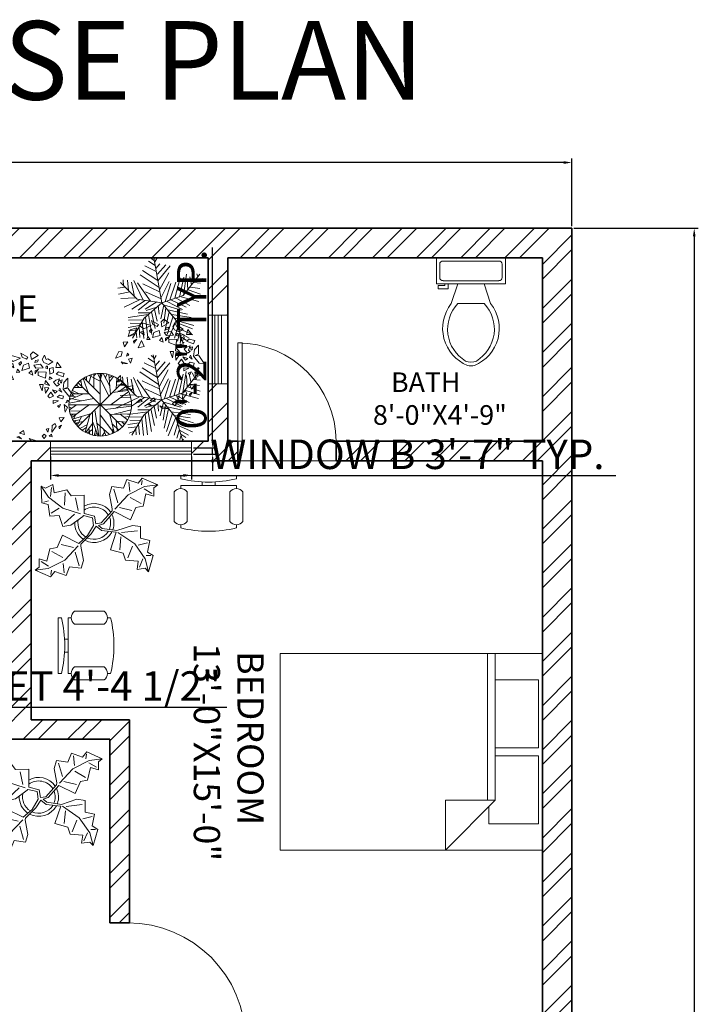
# Model space of a CAD drawing. Units: inches. Extents: x 744 to 1448, y 5126 to 6077.
# Tile 10 of 10: x 1152 to 1359, y 5585 to 5885. Entities that reach past the tile are written whole.
import ezdxf

# ---------------------------------------------------------------- set-up
doc = ezdxf.new("R2010")
doc.units = ezdxf.units.IN
for name, color, linetype, lineweight in [('A-ANNO-DIMS', 2, 'Continuous', 18), ('A-ANNO-TEXT', 7, 'Continuous', 18), ('A-AREA-IDEN', 7, 'Continuous', 18), ('A-DOOR', 4, 'Continuous', 18), ('A-FLOR-FIXT', 9, 'Continuous', 18), ('A-FURN', 8, 'Continuous', 18), ('A-WALL', 7, 'Continuous', 35), ('A-WALL-PATT', 252, 'Continuous', 13), ('L-PLNT', 3, 'Continuous', 13)]:
    doc.layers.add(name, color=color, linetype=linetype, lineweight=lineweight)
doc.layers.add('A-GLAZ', color=244, linetype='Continuous', lineweight=18, true_color=0x991b1e)
doc.styles.get("Standard").update_dxf_attribs({"font": 'arial.ttf'})
doc.dimstyles.new('ISO-25', dxfattribs={"dimtxt": 9, "dimasz": 2.5, "dimexe": 1.25, "dimexo": 0.625, "dimtad": 1, "dimlunit": 3, "dimtxsty": 'Standard', "dimcen": 2.5, "dimadec": 0, "dimazin": 0, "dimtfac": 1, "dimtmove": 0, "dimatfit": 3, "dimfxl": 1, "dimarcsym": 0})

# ---------------------------------------------------------------- blocks, each defined once
blk = doc.blocks.new('*U5')
for p, q in [((0, 0), (0, 6)), ((40, 0), (40, 6))]:
    blk.add_line(p, q)
blk.add_lwpolyline([(0, 0), (0, -40), (1.75, -40), (1.75, 0)], close=True)
blk.add_arc((0, 0), 40, 270, 0)
blk = doc.blocks.new('*U3')
for p, q in [((-40, 0), (-40, 6)), ((0, 0), (0, 6))]:
    blk.add_line(p, q)
blk.add_lwpolyline([(0, 0), (0, -40), (-1.75, -40), (-1.75, 0)], close=True)
blk.add_arc((0, 0), 40, 180, 270)
blk = doc.blocks.new('*U8')
for p, q in [((9.5, -6), (9.5, -2)), ((-10, -8.5), (-8, -8.5)), ((-10, -9.5), (-10, -8.5)), ((-8, -8.5), (-8, -8)), ((-7, -8), (-7, -9.5)), ((-4, -8), (-6, -14)), ((4, -8), (6, -14)), ((-7, -9.5), (-10, -9.5)), ((4, -14), (-4, -14))]:
    blk.add_line(p, q)
blk.add_lwpolyline([(10.5, -8), (10.5, 0), (-10.5, 0), (-10.5, -8)], close=True)
for points in [[(-9.5, -2), (-9.5, -6)], [(8.5, -1), (-8.5, -1)], [(-8.5, -7), (8.5, -7)]]:
    blk.add_lwpolyline(points)
for centre, radius, start, end in [((-8.62, -1.88), 0.884, 81.8699, 188.1301), ((8.62, -1.88), 0.884, 351.8699, 98.1301), ((-8.62, -6.12), 0.884, 171.8699, 278.1301), ((8.62, -6.12), 0.884, 261.8699, 8.1301), ((3.52, -21.58), 12.17, 141.4691, 247.9714), ((4.2, -21.82), 11.33, 136.3677, 238.9468), ((-3.52, -21.58), 12.17, 292.0284, 38.5307), ((-4.2, -21.82), 11.33, 301.053, 43.6321), ((0, -27.88), 4, 245.7318, 294.2682), ((0, -29), 4, 254.8605, 285.1395)]:
    blk.add_arc(centre, radius, start, end)
blk = doc.blocks.new('Bed - Queen')
for p, q in [((0, -80.00003), (0, 0)), ((0, 0), (59.99999, 0)), ((59.99999, 0), (59.99999, -80.00003)), ((7.99999, -1.2), (28.79998, -1.2)), ((7.99999, -14.4), (7.99999, -1.2)), ((28.79998, -1.2), (28.79998, -14.4)), ((31.19999, -1.2), (51.99999, -1.2)), ((31.19999, -14.4), (31.19999, -1.2)), ((51.99999, -1.2), (51.99999, -16.4)), ((0, -14.4), (44.8, -14.4)), ((59.99999, -29.6), (44.8, -14.4)), ((44.8, -14.4), (44.8, -29.6)), ((44.8, -16.8), (0, -16.8)), ((51.99999, -16.4), (46.79936, -16.4)), ((44.8, -29.6), (59.99999, -29.6)), ((59.99999, -80.00003), (0, -80.00003))]:
    blk.add_line(p, q)
blk = doc.blocks.new('Plant - Rubber or Philodendron')
for p, q in [((8.8871, 10.7908), (9.9809, 13.4933)), ((9.9809, 13.4933), (13.3837, 12.301)), ((10.5828, 12.6946), (10.8893, 9.7953)), ((13.3837, 12.301), (14.68, 13.9039)), ((14.5816, 13.2037), (14.3848, 11.8033)), ((14.68, 13.9039), (19.3848, 11.8146)), ((-16.2005, 11.4774), (-13.9899, 8.1064)), ((-16.2005, 11.4774), (-14.8639, 10.7964)), ((-16.0159, 6.3329), (-16.2005, 11.4774)), ((-14.8639, 10.7964), (-12.6195, 11.8975)), ((-13.3174, 8.325), (-13.0735, 11.0065)), ((-12.6195, 11.8975), (-12.1909, 9.4345)), ((-12.1909, 9.4345), (-8.3829, 10.3)), ((-8.8369, 9.409), (-9.0894, 5.6095)), ((-8.3829, 10.3), (-7.0549, 8.501)), ((4.6914, 8.8812), (5.3859, 11.2828)), ((5.3859, 11.2828), (8.8871, 10.7908)), ((5.9878, 10.4842), (7.1971, 6.3869)), ((15.3859, 11.3055), (10.3916, 8.7942)), ((15.7909, 9.1065), (14.8995, 5.3044)), ((15.2875, 10.6053), (17.5907, 9.2105)), ((19.3848, 11.8146), (15.3859, 11.3055)), ((18.1925, 8.4119), (15.7909, 9.1065)), ((19.3848, 11.8146), (18.1868, 10.9119)), ((18.1868, 10.9119), (18.1925, 8.4119)), ((-14.0069, 5.8704), (-16.0159, 6.3329)), ((-15.3434, 6.5514), (-13.9984, 6.9884)), ((-13.9899, 8.1064), (-9.5434, 4.7185)), ((-7.0549, 8.501), (-3.0284, 8.6941)), ((-4.8529, 4.012), (-5.7184, 7.82)), ((-3.0284, 8.6941), (-3.0709, 3.1041)), ((4.6914, 8.8812), (5.5014, 4.4831)), ((10.3916, 8.7942), (6.2847, 4.4028)), ((14.2977, 6.1031), (10.9934, 7.9956)), ((-13.5868, 2.2894), (-14.0069, 5.8704)), ((-13.1329, 3.1804), (-10.6614, 4.727)), ((-9.5434, 4.7185), (-4.1917, 2.9888)), ((-3.0709, 3.1041), (0.0797, 2.3163)), ((2.1141, 0.2298), (5.4346, 3.9146)), ((6.1032, 3.6844), (2.8262, -0.031)), ((5.4346, 3.9146), (5.5014, 4.4831)), ((11.1089, 1.1958), (6.1032, 3.6844)), ((7.7005, 4.8881), (11.5025, 3.9967)), ((12.7005, 4.8994), (11.1089, 1.1958)), ((14.8995, 5.3044), (12.7005, 4.8994)), ((-10.6784, 2.491), (-13.5868, 2.2894)), ((-9.5858, -0.8715), (-10.6784, 2.491)), ((-9.1318, 0.0195), (-5.9793, 2.9025)), ((-7.1228, -0.443), (-3.5248, 2.2131)), ((-3.5248, 2.2131), (-3.3011, 2.4355)), ((-3.3011, 2.4355), (-0.5306, 1.7947)), ((-0.5306, 1.7947), (-0.2255, -0.5527)), ((-0.5306, 1.7947), (-0.5306, 1.7947)), ((0.0797, 2.3163), (0.4866, -0.031)), ((0.4866, -0.031), (2.1141, 0.2298)), ((-7.1228, -0.443), (-9.5858, -0.8715)), ((-2.019, -3.6148), (-0.2255, -0.5527)), ((-0.9375, -3.1608), (0.5883, -0.8135)), ((0.5883, -0.8135), (2.2447, -2.0916)), ((2.8262, -0.031), (1.3003, -0.5527)), ((1.3003, -0.5527), (2.4193, -1.4655)), ((2.2447, -2.0916), (6.7108, -2.6626)), ((2.4193, -1.4655), (6.895, -2.1175)), ((4.943, -7.9659), (6.7108, -2.6626)), ((11.6605, -0.5413), (6.895, -2.1175)), ((12.3677, -6.1981), (7.219, -2.6772)), ((8.3544, -2.7453), (13.1973, -2.1704)), ((11.6605, -0.5413), (14.1354, -0.8948)), ((14.1354, -0.8948), (14.1354, -4.4304)), ((-11.3237, -7.2629), (-9.7321, -3.5593)), ((-9.7321, -3.5593), (-4.7264, -6.0479)), ((-2.019, -3.6148), (-4.7264, -6.0479)), ((-4.0579, -6.2781), (-0.9375, -3.1608)), ((8.125, -4.0768), (7.7715, -7.9659)), ((16.2567, -5.8446), (13.4283, -6.5517)), ((14.1354, -4.4304), (16.9638, -5.1375)), ((16.9638, -5.1375), (16.2567, -8.673)), ((-14.4141, -11.4699), (-13.5228, -7.6679)), ((-13.5228, -7.6679), (-11.3237, -7.2629)), ((-12.921, -8.4665), (-9.6166, -10.359)), ((-6.3237, -7.2516), (-10.1257, -6.3602)), ((-9.0148, -11.1577), (-4.9047, -6.8122)), ((-4.611, -12.8477), (-5.8203, -8.7504)), ((-4.1246, -6.8466), (-4.0579, -6.2781)), ((-3.3146, -11.2447), (-4.1246, -6.8466)), ((8.8321, -9.0266), (4.943, -7.9659)), ((10.2463, -10.4408), (11.6605, -6.9053)), ((15.5496, -10.7943), (12.3677, -6.1981)), ((16.2567, -8.673), (18.0245, -9.7337)), ((-16.8157, -10.7754), (-14.4141, -11.4699)), ((-16.8101, -13.2754), (-16.8157, -10.7754)), ((-13.9107, -12.9688), (-16.2139, -11.574)), ((-14.0091, -13.669), (-9.0148, -11.1577)), ((-3.3146, -11.2447), (-4.0092, -13.6463)), ((9.5392, -11.1479), (8.8321, -9.0266)), ((13.4283, -11.5015), (9.5392, -11.1479)), ((13.0748, -13.9763), (13.4283, -11.5015)), ((14.8425, -10.7943), (13.7819, -13.2692)), ((16.6103, -14.6834), (15.5496, -10.7943)), ((17.3174, -9.7337), (15.9032, -9.7337)), ((18.0245, -9.7337), (16.6103, -14.6834)), ((-18.008, -14.1781), (-16.8101, -13.2754)), ((-18.008, -14.1781), (-14.0091, -13.669)), ((-13.3032, -16.2674), (-18.008, -14.1781)), ((-12.0069, -14.6645), (-13.3032, -16.2674)), ((-13.2048, -15.5672), (-13.008, -14.1668)), ((-8.6042, -15.8568), (-12.0069, -14.6645)), ((-9.206, -15.0581), (-9.5126, -12.1588)), ((-7.5103, -13.1543), (-8.6042, -15.8568)), ((-4.0092, -13.6463), (-7.5103, -13.1543)), ((15.5496, -13.6228), (13.0748, -13.9763)), ((16.6103, -14.6834), (15.5496, -13.6228))]:
    blk.add_line(p, q)
for centre, radius, start, end in [((0, 0), 6.1275, 34.37569, 120.1028), ((-0.0601, -0.2075), 5.2461, 33.82192, 124.9414), ((0.0308, 0.1664), 6, 178.6147, 235.1169), ((0.0308, 0.1664), 5, 168.1647, 238.6725), ((-0.2664, 0.1682), 5.2775, 338.4094, 20.03007), ((-0.098, 0.1364), 6.1288, 341.2017, 26.09184), ((-0.0234, 0.3825), 6.1492, 242.5812, 331.2714), ((-0.1102, 0.4886), 5.2883, 247.3711, 327.472)]:
    blk.add_arc(centre, radius, start, end)
blk = doc.blocks.new('*U11')
for points in [[(-4.43, 11.05), (-5.18, 10.36), (-3.96, 9.49), (-2.07, 10.36)], [(-2, 11.66), (-1.6, 10.62), (-0.52, 10.1), (-0.18, 10.62), (-0.79, 10.96)], [(1.24, 12), (0.56, 11.31), (0.76, 10.01), (2.52, 11.05)], [(4.14, 11.14), (3.6, 10.01), (4, 9.23), (5.22, 8.71), (6.3, 9.41), (5.08, 10.19), (4.61, 10.01)], [(-5.78, 9.75), (-7.54, 9.23), (-8.01, 7.5), (-6.26, 8.45)], [(-4.84, 8.63), (-3.83, 7.85), (-4.03, 8.97)], [(-1.94, 9.49), (-2.48, 8.97), (-2.27, 8.54), (-1.8, 9.06)], [(0.02, 9.06), (-1.33, 8.54), (-1.73, 7.16), (0.29, 7.76)], [(1.37, 8.54), (3.13, 8.8), (3.8, 7.85), (1.91, 7.76)], [(2.59, 9.93), (1.84, 9.75), (1.64, 9.23), (2.32, 9.41)], [(4.61, 8.28), (4.54, 7.76), (4.95, 7.59), (4.95, 8.28)], [(6.43, 7.94), (5.49, 7.68), (5.56, 6.21), (6.5, 6.64)], [(7.45, 9.32), (7.11, 7.94), (8.52, 7.94)], [(-8.14, 6.03), (-9.36, 5.95), (-9.02, 4.73)], [(-5.78, 6.81), (-6.66, 6.21), (-6.52, 5.69)], [(-4.57, 6.38), (-5.45, 4.47), (-3.89, 4.82)], [(-2.88, 7.5), (-3.15, 6.64), (-2.27, 6.72)], [(0.76, 7.16), (0.09, 6.46), (1.1, 5.95)], [(1.71, 6.29), (1.71, 7.07), (2.65, 7.5), (2.11, 6.9)], [(2.52, 6.81), (2.52, 5.86), (4.41, 5.17), (4.61, 6.72)], [(5.49, 5.51), (5.42, 4.82), (6.16, 5.08)], [(7.85, 6.81), (7.18, 6.21), (9, 5.51), (9.33, 6.38)], [(10.28, 5.17), (9.2, 4.04), (9, 2.31), (10.48, 0.49), (11.76, 0.41), (10.35, 2.48), (9.33, 2.4), (10.28, 2.83)], [(-11.32, 1.79), (-9.83, 2.31), (-9.63, 3.44), (-10.44, 3.52)], [(-8.21, 3.09), (-8.48, 2.31), (-7.87, 2.57)], [(3.53, 1.88), (2.86, 3.52), (3.8, 3.52)], [(4.41, 4.56), (4.27, 3.7), (5.49, 3.26)], [(4.27, 2.74), (5.29, 2.66), (4.41, 1.27)], [(8.12, 4.99), (7.11, 4.65), (6.5, 4.13), (7.38, 3.09), (8.12, 3.52), (7.65, 3.87)], [(8.19, 2.57), (7.92, 2.05), (8.66, 1.53)], [(8.73, 4.73), (8.19, 4.56), (8.39, 3.87), (8.59, 4.04)], [(-8.21, 0.41), (-9.43, 0.32), (-9.83, 0.84)], [(-7, 1.79), (-7.94, 1.53), (-7.47, 0.49)], [(5.83, 1.53), (5.02, 0.41), (5.49, -0.02), (6.5, 0.41)], [(7.51, 1.71), (6.91, 1.27), (6.23, 2.14)], [(8.12, 0.75), (7.51, 0.15), (8.93, -0.28), (9.13, 0.49)], [(7.78, -0.8), (6.43, -1.5), (6.43, -0.72)], [(8.32, -1.75), (7.98, -2.53), (7.58, -2.1)], [(9.33, -1.75), (9.54, -3.74), (10.14, -2.53)], [(10.08, -0.63), (9.74, -1.32), (10.48, -0.89)], [(-10.03, -2.71), (-10.64, -3.31), (-10.44, -4.44), (-9.9, -3.49)], [(-8.28, -5.73), (-6.79, -5.3), (-7, -6.51)], [(6.1, -8.94), (6.16, -7.21), (6.91, -6.69), (7.24, -7.38)], [(8.05, -8.07), (8.59, -7.12), (7.92, -7.55)], [(9.33, -5.13), (8.46, -6.25), (7.98, -5.22)], [(-4.84, -8.85), (-4.43, -9.45), (-5.99, -9.8)], [(-2.54, -10.06), (-3.02, -10.23), (-1.8, -10.67)], [(-2.34, -9.2), (-1.26, -8.5), (-0.99, -9.54)], [(4.07, -9.45), (3.53, -9.97), (4.07, -10.58), (4.61, -9.89)], [(5.29, -7.98), (4.61, -8.16), (5.02, -8.94)], [(6.03, -9.45), (5.42, -9.97), (6.16, -10.15)], [(0.22, -10.58), (0.83, -11.27), (2.59, -11.36)]]:
    blk.add_lwpolyline(points, close=True)
blk = doc.blocks.new('*U10')
for p, q in [((-8.737, 47.138), (-17.069, 52.711)), ((-10.186, 53.64), (-13.084, 55.962)), ((0, 0), (-10.5, 57)), ((-9.099, 51.782), (-6.563, 55.962)), ((-5.114, 28.097), (-24.676, 40.636)), ((-7.288, 39.707), (-21.778, 46.673)), ((-7.65, 43.423), (-2.578, 49.46)), ((-5.839, 35.992), (4.667, 48.067)), ((-5.114, 27.632), (10.463, 46.673)), ((-2.941, 16.486), (8.652, 37.85)), ((-31.5, 4.5), (-52.5, 25.5)), ((-48.585, 21.131), (-49.309, 29.026)), ((-43.513, 28.561), (-42.427, 15.558)), ((-38.442, 26.239), (-34.819, 7.663)), ((-35.544, 28.097), (-24.314, 3.947)), ((-14.533, 2.09), (-30.834, 25.31)), ((-3.665, 19.273), (-27.574, 35.527)), ((-1.129, 6.734), (9.014, 26.704)), ((10.101, 3.483), (17.708, 26.239)), ((16.259, 5.805), (23.142, 31.348)), ((22.055, 7.198), (27.489, 32.277)), ((27, 9), (48, 36)), ((27.127, 9.056), (31.112, 35.992)), ((31.836, 30.883), (32.561, 16.486)), ((35.096, 32.741), (37.27, 22.524)), ((38.719, 34.134), (41.979, 28.561)), ((40.53, 25.775), (48.862, 24.846)), ((43.791, 29.954), (51.036, 30.883)), ((44.153, 36.456), (45.239, 32.741)), ((-47.498, 19.737), (-55.83, 18.344)), ((-40.615, 13.7), (-55.105, 10.913)), ((-24.314, 23.917), (-2.941, 13.7)), ((-20.691, 13.7), (-1.129, 4.876)), ((3.942, 1.625), (11.187, 24.381)), ((33.285, 16.486), (48.862, 10.913)), ((36.183, 19.737), (48.137, 17.88)), ((-33.37, 6.269), (-52.207, 5.34)), ((-28.299, 3.483), (-47.86, -5.805)), ((-21.416, 3.018), (-38.079, -8.128)), ((0, 0), (-31.5, 4.5)), ((-15.982, 2.09), (-30.11, -9.521)), ((0, 0), (-22.5, -19.5)), ((-6.563, 1.161), (-21.416, -8.128)), ((0, 0), (27, 9)), ((0, 0), (18, -22.5)), ((6.478, 1.625), (26.04, -8.592)), ((11.187, 3.483), (30.749, -5.805)), ((18.07, 5.805), (35.096, -3.483)), ((24.229, 7.663), (46.688, 1.625)), ((29.662, 12.307), (48.137, 6.269)), ((-6.563, -5.805), (-19.967, -9.985)), ((-13.446, -11.378), (-8.737, -32.741)), ((-9.461, -8.592), (-6.201, -23.453)), ((-4.752, -3.483), (-3.665, -14.629)), ((2.493, -3.019), (-1.491, -20.202)), ((1.769, -2.555), (24.229, -9.521)), ((5.029, -6.27), (2.131, -25.775)), ((9.014, -11.378), (3.58, -35.992)), ((7.565, -9.056), (32.198, -14.629)), ((-17.431, -15.094), (-42.789, -18.809)), ((-24.314, -21.596), (-42.427, -22.06)), ((-22.5, -19.5), (-37.5, -45)), ((-15.257, -12.772), (-30.11, -12.772)), ((-25.038, -23.918), (-22.865, -45.281)), ((-20.691, -18.345), (-17.793, -44.352)), ((-17.069, -15.094), (-12.721, -40.172)), ((14.085, -16.951), (6.478, -40.172)), ((18.07, -22.524), (8.289, -45.745)), ((12.274, -15.094), (36.907, -18.809)), ((16.259, -19.738), (36.183, -22.989)), ((18, -22.5), (27, -52.5)), ((18.433, -22.524), (40.53, -29.026)), ((-28.299, -29.026), (-42.789, -31.348)), ((-30.834, -34.135), (-42.427, -35.528)), ((-26.849, -26.24), (-40.253, -25.775)), ((-32.646, -36.921), (-31.921, -44.352)), ((-29.023, -30.884), (-27.936, -43.887)), ((20.244, -30.419), (15.897, -44.816)), ((19.157, -25.311), (38.719, -33.206)), ((21.331, -32.741), (39.081, -40.636)), ((-34.457, -39.708), (-40.978, -42.494)), ((22.78, -37.85), (19.519, -48.532)), ((22.78, -38.314), (34.372, -44.816)), ((24.591, -45.745), (23.142, -50.854)), ((24.591, -43.423), (30.749, -47.603)), ((26.764, -49.925), (28.213, -50.854))]:
    blk.add_line(p, q)
blk = doc.blocks.new('*U13')
for p, q in [((-22.0458, 42.0753), (-16.5881, 57.6486)), ((-12.5388, 54.9406), (-7.9613, 59.4546)), ((-12.3627, 32.1443), (-12.5388, 58.7776)), ((-5.3205, 59.6806), (16.5105, 16.7963)), ((2.426, 54.9406), (-1.4472, 59.9056)), ((0, 59.9996), (0, -60)), ((0.4894, 48.6208), (3.6584, 59.6806)), ((18.2711, 35.5298), (5.419, 59.6806)), ((9.8203, 51.5549), (12.8133, 58.5516)), ((19.6795, 19.5047), (16.3344, 57.6486)), ((-45.8134, 38.2383), (-40.5318, 33.0471)), ((-43.8768, 36.4326), (-44.405, 40.2696)), ((42, 42), (-42, -42)), ((42, -42), (-42, 42)), ((-40.1797, 44.558), (-36.4825, 43.2038)), ((-37.0107, 47.0408), (-35.25, 35.5298)), ((-32.6092, 50.4264), (-23.2782, 23.5674)), ((-31.2008, 51.1035), (-0.2149, 20.1818)), ((-26.4472, 46.5894), (-26.2712, 53.8116)), ((-21.1656, 55.8436), (-0.0388, 45.0094)), ((17.0387, 51.1035), (23.2006, 55.1666)), ((17.7429, 43.6552), (25.4894, 54.2636)), ((31.6513, 50.8778), (30.2429, 30.5643)), ((31.1232, 42.5267), (35.8767, 48.1693)), ((-32.2571, 20.6333), (-59.1937, 9.348)), ((-56.0247, 20.859), (-20.8134, 20.859)), ((-54.7923, 24.4702), (-47.75, 21.0847)), ((-53.2078, 27.4044), (-40.1797, 20.859)), ((-49.8627, 32.8214), (-32.7853, 32.8214)), ((54.3626, 25.3731), (20.9119, 0.3198)), ((23.3767, 23.3417), (53.3063, 27.4044)), ((36.2288, 25.1474), (48.9049, 35.0784)), ((37.1091, 37.1098), (46.6161, 37.5612)), ((-59.7219, 2.8025), (-12.0106, 12.0565)), ((-58.6656, 12.7336), (-35.9543, 7.5424)), ((-57.081, 17.9248), (-47.0458, 14.7649)), ((-54.6162, -24.7335), (-20.2853, 0.0941)), ((29.3626, -6.6771), (59.4682, 7.091)), ((38.5175, 13.4107), (58.2359, 13.6364)), ((-60, 0), (60, 0)), ((-59.7219, -4.8714), (-54.2641, -6.6771)), ((-45.2853, -0.1316), (-59.0177, -10.0627)), ((-58.4895, -12.3197), (-36.4825, -11.6426)), ((-57.081, -18.4138), (-45.2853, -17.9624)), ((-52.6797, -18.188), (-55.4966, -22.0251)), ((-53.2078, -27.442), (-16.7641, -16.6081)), ((-14.8275, -15.0282), (-14.6515, -57.6865)), ((-10.074, -10.0627), (-2.5036, -59.7178)), ((9.2922, -9.1598), (59.6443, -2.8401)), ((18.6232, -18.6394), (26.7218, -53.3981)), ((18.7992, -18.6394), (57.3556, -17.2853)), ((26.3697, -18.4138), (58.9401, -9.8369)), ((38.1654, -18.188), (52.426, -29.0219)), ((-38.9472, -29.0219), (-51.4472, -30.6018)), ((-47.2219, -19.3166), (-50.2148, -26.3135)), ((-46.5177, -30.1504), (-49.5106, -33.536)), ((-32.4331, -32.4075), (-48.1021, -35.5674)), ((-43.7008, -34.6645), (-46.6937, -37.373)), ((-35.9543, -22.4765), (-44.0529, -40.5329)), ((-19.9331, -20.2194), (-28.5599, -52.721)), ((-14.6515, -36.2445), (-27.6797, -52.9467)), ((-14.6515, -32.1818), (-3.912, -59.4922)), ((-6.2008, -36.2445), (17.919, -57.0094)), ((-0.0388, -19.0909), (25.8415, -53.8495)), ((22.8485, -36.4702), (35.3485, -48.4326)), ((30.419, -30.1504), (32.3556, -50.0125)), ((31.4753, -31.279), (49.6091, -33.3103)), ((41.5105, -32.6332), (46.088, -38.0501)), ((45.9119, -24.0564), (55.595, -22.2508)), ((-24.6867, -37.8244), (-38.7712, -45.7241)), ((-26.2712, -43.9185), (-34.7219, -48.6583)), ((-14.6515, -47.3041), (-25.0388, -54.3009)), ((-21.5177, -45.4984), (-19.9331, -56.1065)), ((-8.4895, -47.5298), (-11.4825, -58.5893)), ((-6.3768, -52.721), (-9.3698, -58.815)), ((8.4119, -53.1724), (3.8344, -59.4922)), ((5.9471, -46.6269), (10.5246, -58.5893)), ((24.7852, -44.8213), (23.0246, -54.978))]:
    blk.add_line(p, q)
blk.add_circle((0, 0), 60)
blk = doc.blocks.new('Chair - Desk')
for p, q in [((-8.5, 0), (-8.5, -1)), ((-8.5, 0), (8.5, 0)), ((8.5, 0), (8.5, -1)), ((-8.5, -3), (-8.5, -4)), ((-8.5, -3), (8.5, -3)), ((-2, -3), (-2, -1.9355)), ((2, -1.9576), (2, -3)), ((8.5, -3), (8.5, -4)), ((-10.5, -5), (-10.5, -14)), ((-6.5, -14), (-6.5, -5)), ((6.5, -5), (6.5, -14)), ((10.5, -14), (10.5, -5)), ((-8.5, -15), (-8.5, -16)), ((8.5, -15), (8.5, -16))]:
    blk.add_line(p, q)
for centre, radius, start, end in [((0, 34.625), 36.625, 256.5803, 283.4197), ((-8.5, -6.5), 2.5, 36.8699, 143.1301), ((8.5, -6.5), 2.5, 36.8699, 143.1301), ((-8.5, -12.5), 2.5, 216.8699, 323.1301), ((8.5, -12.5), 2.5, 216.8699, 323.1301), ((0, 19.625), 36.625, 256.5803, 283.4197)]:
    blk.add_arc(centre, radius, start, end)
blk = doc.blocks.new('*D23')
at = {"layer": 'A-ANNO-DIMS', "color": 0, "lineweight": -2, "transparency": 16777216}
for p, q in [((1321.31, 5821.82), (1359.26, 5821.82)), ((1358.01, 5819.32), (1358.01, 5252.82)), ((1321.31, 5250.32), (1359.26, 5250.32))]:
    blk.add_line(p, q, dxfattribs=at)
at = {"layer": 'A-ANNO-DIMS', "color": 0, "transparency": 16777216}
for points in [[(1357.59, 5819.32), (1358.42, 5819.32), (1358.01, 5821.82)], [(1357.59, 5252.82), (1358.42, 5252.82), (1358.01, 5250.32)]]:
    blk.add_solid(points, dxfattribs=at)
at = {"layer": 'Defpoints', "color": 0, "transparency": 16777216}
for p in [(1320.68, 5821.82), (1320.68, 5250.32), (1358.01, 5250.32)]:
    blk.add_point(p, dxfattribs=at)
at = {"layer": 'A-ANNO-DIMS', "color": 0, "transparency": 16777216, "insert": (1352.81, 5536.07), "char_height": 9, "attachment_point": 5, "rotation": 90}
blk.add_mtext('47\'-7.5"', dxfattribs=at)
blk = doc.blocks.new('*D24')
at = {"layer": 'A-ANNO-DIMS', "color": 0, "lineweight": -2, "transparency": 16777216}
for p, q in [((804.68, 5822.44), (804.68, 5843.13)), ((1320.68, 5822.44), (1320.68, 5843.13)), ((1318.18, 5841.88), (807.18, 5841.88))]:
    blk.add_line(p, q, dxfattribs=at)
at = {"layer": 'A-ANNO-DIMS', "color": 0, "transparency": 16777216}
for points in [[(807.18, 5842.3), (807.18, 5841.46), (804.68, 5841.88)], [(1318.18, 5842.3), (1318.18, 5841.46), (1320.68, 5841.88)]]:
    blk.add_solid(points, dxfattribs=at)
at = {"layer": 'Defpoints', "color": 0, "transparency": 16777216}
for p in [(804.68, 5841.88), (804.68, 5821.82), (1320.68, 5821.82)]:
    blk.add_point(p, dxfattribs=at)
at = {"layer": 'A-ANNO-DIMS', "color": 0, "transparency": 16777216, "insert": (1062.68, 5847.1), "char_height": 9, "attachment_point": 5}
blk.add_mtext("43'", dxfattribs=at)
blk = doc.blocks.new('WINDOW-GLASS-43IN')
for p, q in [((0, 2), (43, 2)), ((0, 1), (43, 1)), ((0, 0), (43, 0))]:
    blk.add_line(p, q)
blk = doc.blocks.new('WINDOW-GLASS-21IN')
for p, q in [((0, 21), (0, 0)), ((1, 21), (1, 0)), ((2, 21), (2, 0))]:
    blk.add_line(p, q)
blk = doc.blocks.new('*D39')
at = {"layer": 'A-ANNO-DIMS', "color": 0, "lineweight": -2, "transparency": 16777216}
for p, q in [((1161.58, 5752.19), (1161.58, 5745.12)), ((1204.58, 5752.19), (1204.58, 5745.12)), ((1164.08, 5746.37), (1202.08, 5746.37)), ((1204.58, 5746.37), (1334.09, 5746.37))]:
    blk.add_line(p, q, dxfattribs=at)
at = {"layer": 'A-ANNO-DIMS', "color": 0, "transparency": 16777216}
for points in [[(1164.08, 5746.78), (1164.08, 5745.95), (1161.58, 5746.37)], [(1202.08, 5746.78), (1202.08, 5745.95), (1204.58, 5746.37)]]:
    blk.add_solid(points, dxfattribs=at)
at = {"layer": 'Defpoints', "color": 0, "transparency": 16777216}
for p in [(1161.58, 5752.82), (1204.58, 5752.82), (1204.58, 5746.37)]:
    blk.add_point(p, dxfattribs=at)
at = {"layer": 'A-ANNO-DIMS', "color": 0, "transparency": 16777216, "insert": (1270.58, 5751.65), "char_height": 9, "attachment_point": 5}
blk.add_mtext('WINDOW B 3\'-7" TYP.', dxfattribs=at)
blk = doc.blocks.new('*D40')
at = {"layer": 'A-ANNO-DIMS', "color": 0, "lineweight": -2, "transparency": 16777216}
for p, q in [((1211.03, 5757.32), (1211.03, 5815.93)), ((1205.2, 5754.82), (1212.28, 5754.82)), ((1205.2, 5752.82), (1212.28, 5752.82)), ((1211.03, 5752.82), (1211.03, 5754.82)), ((1211.03, 5750.32), (1211.03, 5747.82))]:
    blk.add_line(p, q, dxfattribs=at)
at = {"layer": 'A-ANNO-DIMS', "color": 0, "transparency": 16777216}
for points in [[(1210.61, 5757.32), (1211.44, 5757.32), (1211.03, 5754.82)], [(1210.61, 5750.32), (1211.44, 5750.32), (1211.03, 5752.82)]]:
    blk.add_solid(points, dxfattribs=at)
at = {"layer": 'Defpoints', "color": 0, "transparency": 16777216}
for p in [(1204.58, 5754.82), (1204.58, 5752.82), (1211.03, 5754.82)]:
    blk.add_point(p, dxfattribs=at)
at = {"layer": 'A-ANNO-DIMS', "color": 0, "transparency": 16777216, "insert": (1205.81, 5787.87), "char_height": 9, "attachment_point": 5, "rotation": 90}
blk.add_mtext('0\'-2" TYP.', dxfattribs=at)
blk = doc.blocks.new('*D47')
at = {"layer": 'A-ANNO-DIMS', "color": 0, "lineweight": -2, "transparency": 16777216}
for p, q in [((1039.05, 5682.9), (1039.05, 5674.38)), ((1091.7, 5682.9), (1091.7, 5674.38)), ((1041.55, 5675.63), (1089.2, 5675.63)), ((1091.7, 5675.63), (1215.34, 5675.63))]:
    blk.add_line(p, q, dxfattribs=at)
at = {"layer": 'A-ANNO-DIMS', "color": 0, "transparency": 16777216}
for points in [[(1041.55, 5676.05), (1041.55, 5675.22), (1039.05, 5675.63)], [(1089.2, 5676.05), (1089.2, 5675.22), (1091.7, 5675.63)]]:
    blk.add_solid(points, dxfattribs=at)
at = {"layer": 'Defpoints', "color": 0, "transparency": 16777216}
for p in [(1039.05, 5683.53), (1091.7, 5683.53), (1091.7, 5675.63)]:
    blk.add_point(p, dxfattribs=at)
at = {"layer": 'A-ANNO-DIMS', "color": 0, "transparency": 16777216, "insert": (1154.77, 5680.91), "char_height": 9, "attachment_point": 5}
blk.add_mtext('DINING SET 4\'-4 1/2"', dxfattribs=at)
blk = doc.blocks.new('*D58')
at = {"layer": 'A-ANNO-DIMS', "color": 0, "lineweight": -2, "transparency": 16777216}
for p, q in [((1128.86, 5714.27), (1128.86, 5125.91)), ((1146.83, 5714.27), (1146.83, 5125.91)), ((1131.36, 5127.16), (1144.33, 5127.16)), ((1146.83, 5127.16), (1173.66, 5127.16))]:
    blk.add_line(p, q, dxfattribs=at)
at = {"layer": 'A-ANNO-DIMS', "color": 0, "transparency": 16777216}
for points in [[(1131.36, 5127.58), (1131.36, 5126.75), (1128.86, 5127.16)], [(1144.33, 5127.58), (1144.33, 5126.75), (1146.83, 5127.16)]]:
    blk.add_solid(points, dxfattribs=at)
at = {"layer": 'Defpoints', "color": 0, "transparency": 16777216}
for p in [(1128.86, 5714.9), (1146.83, 5714.9), (1146.83, 5127.16)]:
    blk.add_point(p, dxfattribs=at)
at = {"layer": 'A-ANNO-DIMS', "color": 0, "transparency": 16777216, "insert": (1161.49, 5132.38), "char_height": 9, "attachment_point": 5}
blk.add_mtext('1\'-6"', dxfattribs=at)

msp = doc.modelspace()

# ---------------------------------------------------------------- hatches: boundary and pattern name
at = {"layer": 'A-WALL-PATT'}
h = msp.add_hatch(dxfattribs=at)
h.set_pattern_fill('ANSI32', color=256)
h.paths.add_polyline_path([(813.684, 5750.816), (876.684, 5750.816), (876.684, 5756.816), (813.684, 5756.816), (813.684, 5812.816), (909.684, 5812.816), (909.684, 5795.316), (915.684, 5795.316), (915.684, 5812.816), (1209.684, 5812.816), (1209.684, 5795.316), (1215.684, 5795.316), (1215.684, 5812.816), (1311.684, 5812.816), (1311.684, 5756.816), (1248.684, 5756.816), (1248.684, 5750.816), (1311.684, 5750.816), (1311.684, 5570.816), (1179.044, 5570.816), (1179.044, 5564.816), (1311.684, 5564.816), (1311.684, 5383.316), (1260.684, 5383.316), (1260.684, 5377.316), (1311.684, 5377.316), (1311.684, 5320.316), (1227.684, 5320.316), (1227.684, 5333.816), (1221.684, 5333.816), (1221.684, 5314.316), (1320.684, 5314.316), (1320.684, 5821.816), (804.684, 5821.816), (804.684, 5472.316), (926.184, 5472.316), (926.184, 5481.316), (813.684, 5481.316), (813.684, 5581.616), (946.284, 5581.616), (946.284, 5587.616), (813.684, 5587.616)])
h.paths.add_polyline_path([(1155.684, 5525.816), (1149.684, 5525.816), (1149.684, 5481.316), (1025.184, 5481.316), (1025.184, 5475.316), (1146.684, 5475.316), (1146.684, 5323.316), (1118.788, 5323.316), (1118.788, 5314.316), (1146.684, 5314.316), (1155.684, 5314.316), (1155.684, 5374.316), (1170.35, 5374.316), (1170.35, 5383.316), (1155.684, 5383.316)], flags=17)
h.paths.add_polyline_path([(1230.684, 5383.316), (1213.35, 5383.316), (1213.35, 5374.316), (1221.684, 5374.316), (1221.684, 5363.816), (1226.184, 5363.816), (1227.684, 5363.816), (1227.684, 5377.316), (1230.684, 5377.316)], flags=17)
h.paths.add_polyline_path([(1185.684, 5671.816), (1155.684, 5671.816), (1155.684, 5750.816), (1161.575, 5750.816), (1161.575, 5756.816), (1157.542, 5756.816), (1157.847, 5756.715), (1155.79, 5756.816), (1149.684, 5756.816), (1149.684, 5750.816), (1149.684, 5671.816), (1121.684, 5671.816), (1121.684, 5665.816), (1179.684, 5665.816), (1179.684, 5609.816), (1185.684, 5609.816)], flags=17)
h.paths.add_polyline_path([(1003.684, 5671.816), (975.684, 5671.816), (975.684, 5750.816), (975.684, 5756.816), (965.205, 5756.816), (965.205, 5750.816), (969.684, 5750.816), (969.684, 5671.816), (939.684, 5671.816), (939.684, 5626.616), (945.684, 5626.616), (945.684, 5665.816), (1003.684, 5665.816)], flags=17)
h.paths.add_polyline_path([(915.684, 5774.316), (909.684, 5774.316), (909.684, 5756.816), (906.684, 5756.816), (906.684, 5752.316), (906.684, 5750.816), (922.205, 5750.816), (922.205, 5756.816), (915.684, 5756.816)], flags=17)
h.paths.add_polyline_path([(1215.684, 5774.316), (1209.684, 5774.316), (1209.684, 5756.816), (1204.575, 5756.816), (1204.575, 5750.816), (1218.684, 5750.816), (1218.684, 5756.816), (1215.684, 5756.816)], flags=17)
h.paths.add_polyline_path([(1063.788, 5323.316), (1025.184, 5323.316), (1025.184, 5314.316), (1063.788, 5314.316)])
h.paths.add_polyline_path([(986.184, 5475.316), (989.184, 5475.316), (989.184, 5481.316), (974.184, 5481.316), (974.184, 5475.916), (974.184, 5472.316), (977.184, 5472.316), (977.184, 5314.316), (989.184, 5314.316), (989.184, 5319.716), (989.184, 5323.316), (986.184, 5323.316)])

# ---------------------------------------------------------------- linework, layer by layer
at = {"layer": 'A-DOOR'}
msp.add_line((1218.684, 5750.816), (1248.684, 5750.816), dxfattribs=at)
at = {"layer": 'A-GLAZ'}
for points in [[(1209.684, 5795.316), (1215.684, 5795.316), (1215.684, 5774.316), (1209.684, 5774.316)], [(1161.575, 5756.816), (1204.575, 5756.816), (1204.575, 5750.816), (1161.575, 5750.816)]]:
    msp.add_lwpolyline(points, close=True, dxfattribs=at)
at = {"layer": 'A-WALL'}
for p, q in [((804.684, 5821.816), (1320.684, 5821.816)), ((1320.684, 5250.316), (1320.684, 5821.816)), ((915.684, 5812.816), (1209.684, 5812.816)), ((1209.684, 5756.816), (1209.684, 5812.816)), ((1215.684, 5756.816), (1215.684, 5812.816)), ((1215.684, 5812.816), (1311.684, 5812.816)), ((1311.684, 5756.816), (1311.684, 5812.816)), ((1086.684, 5756.816), (1209.684, 5756.816)), ((1215.684, 5756.816), (1218.684, 5756.816)), ((1218.684, 5756.816), (1218.684, 5750.816)), ((1248.684, 5756.816), (1311.684, 5756.816)), ((1248.684, 5756.816), (1248.684, 5750.816)), ((1155.684, 5750.816), (1218.684, 5750.816)), ((1155.684, 5671.816), (1155.684, 5750.816)), ((1248.684, 5750.816), (1311.684, 5750.816)), ((1311.684, 5570.816), (1311.684, 5750.816)), ((1155.684, 5671.816), (1185.684, 5671.816)), ((1185.684, 5609.816), (1185.684, 5671.816)), ((1121.684, 5665.816), (1179.684, 5665.816)), ((1179.684, 5609.816), (1179.684, 5665.816)), ((1185.684, 5609.816), (1179.684, 5609.816))]:
    msp.add_line(p, q, dxfattribs=at)

# ---------------------------------------------------------------- block references
at = {"layer": 'A-DOOR'}
for name, p, xscale, yscale, zscale, rotation in [('*U3', (1218.684, 5756.816), 0.75, 0.75, 0.75, 180.0000000000004), ('*U5', (1185.084, 5573.816), 0.9, 0.9, 0.9, 90)]:
    msp.add_blockref(name, p, dxfattribs=dict(at, xscale=xscale, yscale=yscale, zscale=zscale, rotation=rotation))
at = {"layer": 'A-FLOR-FIXT'}
msp.add_blockref('*U8', (1289.877, 5812.816), dxfattribs=at)
at = {"layer": 'A-FURN'}
msp.add_blockref('Chair - Desk', (1209.783, 5746.329), dxfattribs=at)
for name, p, rotation in [('Chair - Desk', (1163.895, 5694.425), 90), ('Bed - Queen', (1311.684, 5692.016), 270)]:
    msp.add_blockref(name, p, dxfattribs=dict(at, rotation=rotation))
at = {"layer": 'A-GLAZ', "rotation": 180}
msp.add_blockref('WINDOW-GLASS-21IN', (1213.684, 5795.316), dxfattribs=at)
at = {"layer": 'A-GLAZ'}
msp.add_blockref('WINDOW-GLASS-43IN', (1161.575, 5752.816), dxfattribs=at)
at = {"layer": 'L-PLNT'}
for name, p, xscale, yscale, zscale in [('*U10', (1195.568, 5799.083), 0.2409161369388113, 0.2409161369388113, 0.2409161369388113), ('*U11', (1194.669, 5780.026), 1.172842970614158, 1.172842970614158, 1.172842970614158), ('*U11', (1154.815, 5770.036), 1.172842970614158, 1.172842970614158, 1.172842970614158), ('*U10', (1195.417, 5769.462), 0.2409161369388113, 0.2409161369388113, 0.2409161369388113), ('*U13', (1176.725, 5767.957), 0.1595845373812122, 0.1595845373812122, 0.1595845373812122)]:
    msp.add_blockref(name, p, dxfattribs=dict(at, xscale=xscale, yscale=yscale, zscale=zscale))
for p in [(1174.887, 5731.662), (1157.959, 5648.06)]:
    msp.add_blockref('Plant - Rubber or Philodendron', p, dxfattribs=at)

# ---------------------------------------------------------------- texts
at = {"layer": 'A-ANNO-TEXT', "insert": (818.158, 5885.054), "char_height": 24, "attachment_point": 1}
msp.add_mtext_dynamic_manual_height_columns('GROUND FLOOR HOUSE PLAN', width=502.97243, gutter_width=12.5, heights=[0], dxfattribs=at)
at = {"layer": 'A-AREA-IDEN', "attachment_point": 1}
for s, width, insert, char_height in [('OPEN TO SKY FOR LAUNDRY 4\'-5" WIDE', 218.47208, (959.254, 5801.351), 8), ('   BATH\\P8\'-0"X4\'-9"', 39.96322, (1259.964, 5777.819), 6)]:
    msp.add_mtext_dynamic_manual_height_columns(s, width=width, gutter_width=12.5, heights=[0], dxfattribs=dict(at, insert=insert, char_height=char_height))
at = {"layer": 'A-AREA-IDEN', "insert": (1226.611, 5695.171), "char_height": 8, "attachment_point": 1, "rotation": 270}
msp.add_mtext_dynamic_manual_height_columns(' BEDROOM\\P13\'-0"X15\'-0"', width=64.21152, gutter_width=12.5, heights=[0], dxfattribs=at)

# ---------------------------------------------------------------- dimensions: what is measured, and where the dimension line sits
at = {"layer": 'A-ANNO-DIMS'}
for base, p1, p2, override, picture, middle in [((804.684, 5841.882), (1320.684, 5821.816), (804.684, 5821.816), {"dimclrd": 0, "dimclre": 0, "dimclrt": 0}, '*D24', (1062.684, 5847.105)), ((1146.829, 5127.162), (1128.864, 5714.896), (1146.829, 5714.896), {"dimdec": 1, "dimlfac": 1, "dimrnd": 0, "dimzin": 1, "dimdsep": 46, "dimlunit": 4, "dimfrac": 2}, '*D58', (1161.493, 5132.383))]:
    dim = msp.add_linear_dim(base=base, p1=p1, p2=p2, dimstyle='ISO-25', override=override, dxfattribs=at)
    dim.commit()
    dim.dimension.update_dxf_attribs({"geometry": picture, "text_midpoint": middle})
dim = msp.add_linear_dim(base=(1358.008, 5250.316), p1=(1320.684, 5821.816), p2=(1320.684, 5250.316), angle=90, dimstyle='ISO-25', override={"dimclrd": 0, "dimclre": 0, "dimclrt": 0}, dxfattribs=at)
dim.commit()
dim.dimension.update_dxf_attribs({"geometry": '*D23', "text_midpoint": (1352.806, 5536.066)})
dim = msp.add_linear_dim(base=(1211.025, 5754.816), p1=(1204.575, 5752.816), p2=(1204.575, 5754.816), angle=90, text='<> TYP.', dimstyle='ISO-25', override={"dimdec": 1, "dimlfac": 1, "dimrnd": 0, "dimzin": 1, "dimdsep": 46, "dimlunit": 4, "dimfrac": 2}, dxfattribs=at)
dim.commit()
dim.dimension.update_dxf_attribs({"geometry": '*D40', "text_midpoint": (1205.805, 5787.87)})
for base, p1, p2, text, picture, middle in [((1204.575, 5746.366), (1161.575, 5752.816), (1204.575, 5752.816), 'WINDOW B <> TYP.', '*D39', (1270.584, 5751.65)), ((1091.7, 5675.632), (1039.048, 5683.53), (1091.7, 5683.53), 'DINING SET <>', '*D47', (1154.77, 5680.91))]:
    dim = msp.add_linear_dim(base=base, p1=p1, p2=p2, text=text, dimstyle='ISO-25', override={"dimdec": 1, "dimlfac": 1, "dimrnd": 0, "dimzin": 1, "dimdsep": 46, "dimlunit": 4, "dimfrac": 2}, dxfattribs=at)
    dim.commit()
    dim.dimension.update_dxf_attribs({"geometry": picture, "text_midpoint": middle})

doc.saveas('drawing.dxf')
